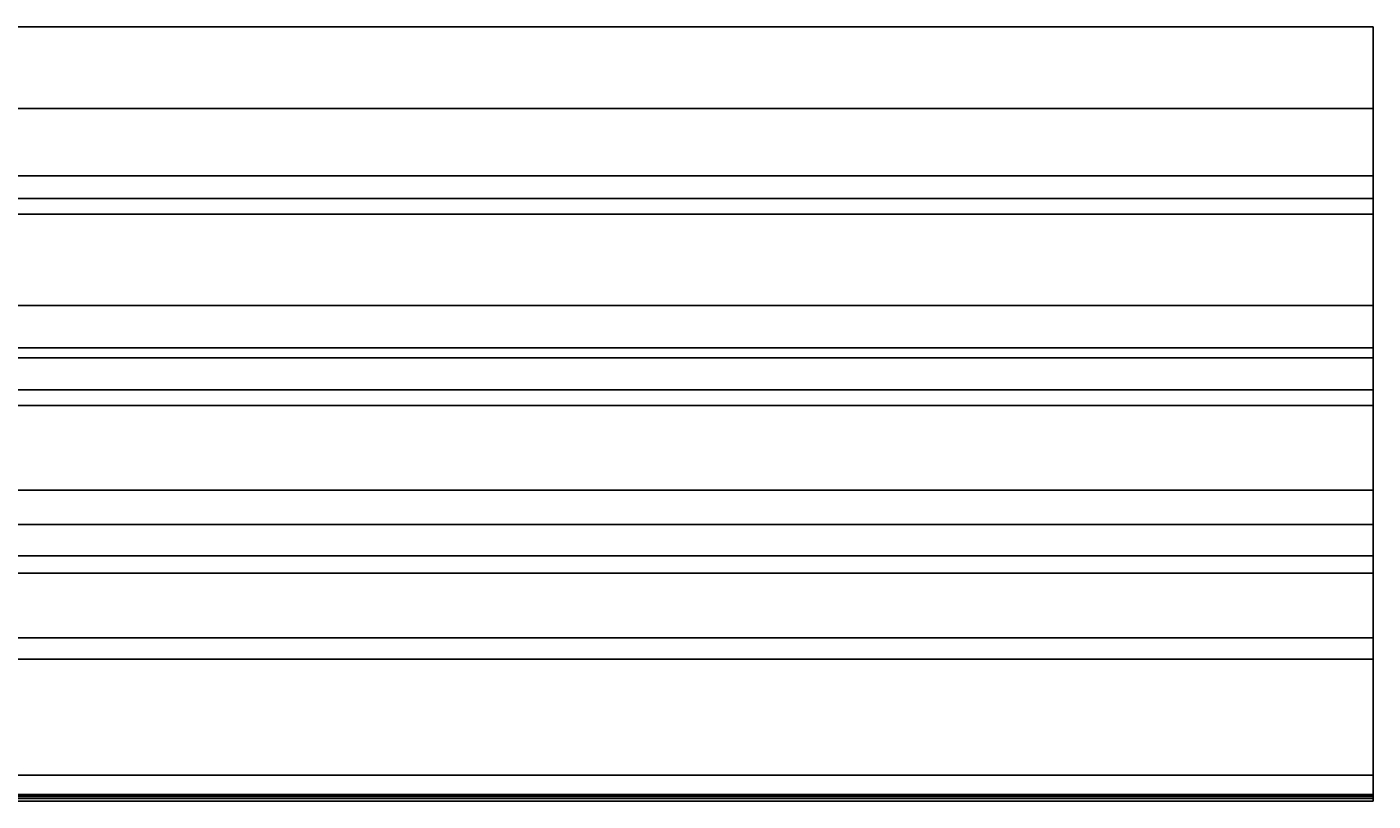
# Model space of a CAD drawing. Units: inches. Extents: x -32109 to 33221, y -19197 to 7608.
# Tile 25 of 25: x 19011 to 25711, y -2148 to 1705. Entities that reach past the tile are written whole.
import ezdxf

# ---------------------------------------------------------------- set-up
doc = ezdxf.new("R2010")
doc.units = ezdxf.units.IN
doc.header["$MEASUREMENT"] = 0
doc.layers.add('A-ANNO-DIMS', color=2, linetype='Continuous', lineweight=18)
doc.layers.add('A-ELEV', color=7, linetype='Continuous', lineweight=25)
doc.styles.get("Standard").update_dxf_attribs({"font": 'arial.ttf'})
doc.dimstyles.get("Standard").update_dxf_attribs({"dimtxt": 0.18, "dimasz": 0.18, "dimexe": 0.18, "dimexo": 0.0625, "dimgap": 0.09, "dimtad": 0, "dimtih": 1, "dimtoh": 1, "dimdec": 4, "dimzin": 0, "dimdsep": 46, "dimtxsty": 'Standard', "dimcen": 0.09, "dimadec": 0, "dimazin": 0, "dimtfac": 1, "dimtdec": 4, "dimtofl": 0, "dimtmove": 0, "dimatfit": 3, "dimfxl": 1, "dimtolj": 1, "dimtzin": 0, "dimarcsym": 0})

# ---------------------------------------------------------------- blocks, each defined once
blk = doc.blocks.new('*D11')
at = {"layer": 'A-ANNO-DIMS', "color": 0, "lineweight": -2, "transparency": 16777216}
for p, q in [((14509.6, 1705.2), (25710.6, 1705.2)), ((25710.5, 1705), (25710.5, -209.6)), ((25710.5, -2124.6), (25710.5, -210)), ((-18512.6, -2124.8), (25710.6, -2124.8))]:
    blk.add_line(p, q, dxfattribs=at)
at = {"layer": 'A-ANNO-DIMS', "color": 0, "transparency": 16777216}
for points in [[(25710.4, 1705), (25710.5, 1705), (25710.5, 1705.2)], [(25710.4, -2124.6), (25710.5, -2124.6), (25710.5, -2124.8)]]:
    blk.add_solid(points, dxfattribs=at)
at = {"layer": 'Defpoints', "color": 0, "transparency": 16777216}
for p in [(14509.6, 1705.2), (-18512.6, -2124.8), (25710.5, -2124.8)]:
    blk.add_point(p, dxfattribs=at)
at = {"layer": 'A-ANNO-DIMS', "color": 0, "transparency": 16777216, "insert": (25710.5, -209.8), "char_height": 0.18, "attachment_point": 5}
blk.add_mtext('\\A1;3830', dxfattribs=at)
blk = doc.blocks.new('*D53')
at = {"layer": 'A-ANNO-DIMS', "color": 0, "lineweight": -2, "transparency": 16777216}
for p, q in [((-9508.3, -179.7), (25710.6, -179.7)), ((25710.5, -179.9), (25710.5, -389.7)), ((25710.5, -600), (25710.5, -390.1)), ((-9508.3, -600.2), (25710.6, -600.2))]:
    blk.add_line(p, q, dxfattribs=at)
at = {"layer": 'A-ANNO-DIMS', "color": 0, "transparency": 16777216}
for points in [[(25710.4, -179.9), (25710.5, -179.9), (25710.5, -179.7)], [(25710.4, -600), (25710.5, -600), (25710.5, -600.2)]]:
    blk.add_solid(points, dxfattribs=at)
at = {"layer": 'Defpoints', "color": 0, "transparency": 16777216}
for p in [(-9508.3, -179.7), (-9508.3, -600.2), (25710.5, -600.2)]:
    blk.add_point(p, dxfattribs=at)
at = {"layer": 'A-ANNO-DIMS', "color": 0, "transparency": 16777216, "insert": (25710.5, -389.9), "char_height": 0.18, "attachment_point": 5}
blk.add_mtext('\\A1;420.5', dxfattribs=at)
blk = doc.blocks.new('*D54')
at = {"layer": 'A-ANNO-DIMS', "color": 0, "lineweight": -2, "transparency": 16777216}
for p, q in [((-9508.3, -600.2), (25710.6, -600.2)), ((25710.5, -600.3), (25710.5, -806.8)), ((25710.5, -1013.7), (25710.5, -807.2)), ((-9508.3, -1013.9), (25710.6, -1013.9))]:
    blk.add_line(p, q, dxfattribs=at)
at = {"layer": 'A-ANNO-DIMS', "color": 0, "transparency": 16777216}
for points in [[(25710.4, -600.3), (25710.5, -600.3), (25710.5, -600.2)], [(25710.4, -1013.7), (25710.5, -1013.7), (25710.5, -1013.9)]]:
    blk.add_solid(points, dxfattribs=at)
at = {"layer": 'Defpoints', "color": 0, "transparency": 16777216}
for p in [(-9508.3, -600.2), (-9508.3, -1013.9), (25710.5, -1013.9)]:
    blk.add_point(p, dxfattribs=at)
at = {"layer": 'A-ANNO-DIMS', "color": 0, "transparency": 16777216, "insert": (25710.5, -807), "char_height": 0.18, "attachment_point": 5}
blk.add_mtext('\\A1;413.7', dxfattribs=at)
blk = doc.blocks.new('*D55')
at = {"layer": 'A-ANNO-DIMS', "color": 0, "lineweight": -2, "transparency": 16777216}
for p, q in [((-9508.3, -1013.9), (25710.6, -1013.9)), ((25710.5, -1014.1), (25710.5, -1227.7)), ((25710.5, -1441.6), (25710.5, -1228)), ((-9508.3, -1441.8), (25710.6, -1441.8))]:
    blk.add_line(p, q, dxfattribs=at)
at = {"layer": 'A-ANNO-DIMS', "color": 0, "transparency": 16777216}
for points in [[(25710.4, -1014.1), (25710.5, -1014.1), (25710.5, -1013.9)], [(25710.4, -1441.6), (25710.5, -1441.6), (25710.5, -1441.8)]]:
    blk.add_solid(points, dxfattribs=at)
at = {"layer": 'Defpoints', "color": 0, "transparency": 16777216}
for p in [(-9508.3, -1013.9), (-9508.3, -1441.8), (25710.5, -1441.8)]:
    blk.add_point(p, dxfattribs=at)
at = {"layer": 'A-ANNO-DIMS', "color": 0, "transparency": 16777216, "insert": (25710.5, -1227.9), "char_height": 0.18, "attachment_point": 5}
blk.add_mtext('\\A1;427.9', dxfattribs=at)
blk = doc.blocks.new('*D56')
at = {"layer": 'A-ANNO-DIMS', "color": 0, "lineweight": -2, "transparency": 16777216}
for p, q in [((-9508.3, -1441.8), (25710.6, -1441.8)), ((25710.5, -1442), (25710.5, -1730.1)), ((25710.5, -2018.6), (25710.5, -1730.5)), ((-9508.3, -2018.8), (25710.6, -2018.8))]:
    blk.add_line(p, q, dxfattribs=at)
at = {"layer": 'A-ANNO-DIMS', "color": 0, "transparency": 16777216}
for points in [[(25710.4, -1442), (25710.5, -1442), (25710.5, -1441.8)], [(25710.4, -2018.6), (25710.5, -2018.6), (25710.5, -2018.8)]]:
    blk.add_solid(points, dxfattribs=at)
at = {"layer": 'Defpoints', "color": 0, "transparency": 16777216}
for p in [(-9508.3, -1441.8), (-9508.3, -2018.8), (25710.5, -2018.8)]:
    blk.add_point(p, dxfattribs=at)
at = {"layer": 'A-ANNO-DIMS', "color": 0, "transparency": 16777216, "insert": (25710.5, -1730.3), "char_height": 0.18, "attachment_point": 5}
blk.add_mtext('\\A1;576.9', dxfattribs=at)
blk = doc.blocks.new('*D67')
at = {"layer": 'A-ANNO-DIMS', "color": 0, "lineweight": -2, "transparency": 16777216}
for p, q in [((1645.9, 851.2), (25710.6, 851.2)), ((25710.5, 851), (25710.5, -632.3)), ((25710.5, -2116), (25710.5, -632.7)), ((1588.2, -2116.1), (25710.6, -2116.1))]:
    blk.add_line(p, q, dxfattribs=at)
at = {"layer": 'A-ANNO-DIMS', "color": 0, "transparency": 16777216}
for points in [[(25710.4, 851), (25710.5, 851), (25710.5, 851.2)], [(25710.4, -2116), (25710.5, -2116), (25710.5, -2116.1)]]:
    blk.add_solid(points, dxfattribs=at)
at = {"layer": 'Defpoints', "color": 0, "transparency": 16777216}
for p in [(1645.8, 851.2), (1588.2, -2116.1), (25710.5, -2116.1)]:
    blk.add_point(p, dxfattribs=at)
at = {"layer": 'A-ANNO-DIMS', "color": 0, "transparency": 16777216, "insert": (25710.5, -632.5), "char_height": 0.18, "attachment_point": 5}
blk.add_mtext('\\A1;2967.4', dxfattribs=at)
blk = doc.blocks.new('*D68')
at = {"layer": 'A-ANNO-DIMS', "color": 0, "lineweight": -2, "transparency": 16777216}
for p, q in [((4084.1, -927.5), (25710.6, -927.5)), ((25710.5, -927.7), (25710.5, -1521.6)), ((25710.5, -2116), (25710.5, -1522)), ((4084.1, -2116.1), (25710.6, -2116.1))]:
    blk.add_line(p, q, dxfattribs=at)
at = {"layer": 'A-ANNO-DIMS', "color": 0, "transparency": 16777216}
for points in [[(25710.4, -927.7), (25710.5, -927.7), (25710.5, -927.5)], [(25710.4, -2116), (25710.5, -2116), (25710.5, -2116.1)]]:
    blk.add_solid(points, dxfattribs=at)
at = {"layer": 'Defpoints', "color": 0, "transparency": 16777216}
for p in [(4084, -927.5), (4084, -2116.1), (25710.5, -2116.1)]:
    blk.add_point(p, dxfattribs=at)
at = {"layer": 'A-ANNO-DIMS', "color": 0, "transparency": 16777216, "insert": (25710.5, -1521.8), "char_height": 0.18, "attachment_point": 5}
blk.add_mtext('\\A1;1188.7', dxfattribs=at)
blk = doc.blocks.new('*D69')
at = {"layer": 'A-ANNO-DIMS', "color": 0, "lineweight": -2, "transparency": 16777216}
for p, q in [((5273.8, 1298.7), (25710.6, 1298.7)), ((25710.5, 1298.5), (25710.5, -411.9)), ((25710.5, -2122.6), (25710.5, -412.2)), ((5279.3, -2122.7), (25710.6, -2122.7))]:
    blk.add_line(p, q, dxfattribs=at)
at = {"layer": 'A-ANNO-DIMS', "color": 0, "transparency": 16777216}
for points in [[(25710.4, 1298.5), (25710.5, 1298.5), (25710.5, 1298.7)], [(25710.4, -2122.6), (25710.5, -2122.6), (25710.5, -2122.7)]]:
    blk.add_solid(points, dxfattribs=at)
at = {"layer": 'Defpoints', "color": 0, "transparency": 16777216}
for p in [(5273.7, 1298.7), (5279.3, -2122.7), (25710.5, -2122.7)]:
    blk.add_point(p, dxfattribs=at)
at = {"layer": 'A-ANNO-DIMS', "color": 0, "transparency": 16777216, "insert": (25710.5, -412), "char_height": 0.18, "attachment_point": 5}
blk.add_mtext('\\A1;3421.4', dxfattribs=at)
blk = doc.blocks.new('*D70')
at = {"layer": 'A-ANNO-DIMS', "color": 0, "lineweight": -2, "transparency": 16777216}
for p, q in [((8883.3, 57.8), (25710.6, 57.8)), ((25710.5, 57.6), (25710.5, -1045.1)), ((25710.5, -2148.2), (25710.5, -1045.5)), ((8832.4, -2148.4), (25710.6, -2148.4))]:
    blk.add_line(p, q, dxfattribs=at)
at = {"layer": 'A-ANNO-DIMS', "color": 0, "transparency": 16777216}
for points in [[(25710.4, 57.6), (25710.5, 57.6), (25710.5, 57.8)], [(25710.4, -2148.2), (25710.5, -2148.2), (25710.5, -2148.4)]]:
    blk.add_solid(points, dxfattribs=at)
at = {"layer": 'Defpoints', "color": 0, "transparency": 16777216}
for p in [(8883.2, 57.8), (8832.3, -2148.4), (25710.5, -2148.4)]:
    blk.add_point(p, dxfattribs=at)
at = {"layer": 'A-ANNO-DIMS', "color": 0, "transparency": 16777216, "insert": (25710.5, -1045.3), "char_height": 0.18, "attachment_point": 5}
blk.add_mtext('\\A1;2206', dxfattribs=at)
blk = doc.blocks.new('*D71')
at = {"layer": 'A-ANNO-DIMS', "color": 0, "lineweight": -2, "transparency": 16777216}
for p, q in [((11823.3, 772.8), (25710.6, 772.8)), ((25710.5, 772.6), (25710.5, 440.5)), ((25710.5, 107.9), (25710.5, 440.1)), ((11823.3, 107.7), (25710.6, 107.7))]:
    blk.add_line(p, q, dxfattribs=at)
at = {"layer": 'A-ANNO-DIMS', "color": 0, "transparency": 16777216}
for points in [[(25710.4, 772.6), (25710.5, 772.6), (25710.5, 772.8)], [(25710.4, 107.9), (25710.5, 107.9), (25710.5, 107.7)]]:
    blk.add_solid(points, dxfattribs=at)
at = {"layer": 'Defpoints', "color": 0, "transparency": 16777216}
for p in [(11823.2, 772.8), (11823.2, 107.7), (25710.5, 107.7)]:
    blk.add_point(p, dxfattribs=at)
at = {"layer": 'A-ANNO-DIMS', "color": 0, "transparency": 16777216, "insert": (25710.5, 440.3), "char_height": 0.18, "attachment_point": 5}
blk.add_mtext('\\A1;665.1', dxfattribs=at)
blk = doc.blocks.new('*D72')
at = {"layer": 'A-ANNO-DIMS', "color": 0, "lineweight": -2, "transparency": 16777216}
for p, q in [((11823.3, 107.7), (25710.6, 107.7)), ((25710.5, 107.6), (25710.5, -1004)), ((25710.5, -2116), (25710.5, -1004.4)), ((11383.7, -2116.1), (25710.6, -2116.1))]:
    blk.add_line(p, q, dxfattribs=at)
at = {"layer": 'A-ANNO-DIMS', "color": 0, "transparency": 16777216}
for points in [[(25710.4, 107.6), (25710.5, 107.6), (25710.5, 107.7)], [(25710.4, -2116), (25710.5, -2116), (25710.5, -2116.1)]]:
    blk.add_solid(points, dxfattribs=at)
at = {"layer": 'Defpoints', "color": 0, "transparency": 16777216}
for p in [(11823.2, 107.7), (11383.7, -2116.1), (25710.5, -2116.1)]:
    blk.add_point(p, dxfattribs=at)
at = {"layer": 'A-ANNO-DIMS', "color": 0, "transparency": 16777216, "insert": (25710.5, -1004.2), "char_height": 0.18, "attachment_point": 5}
blk.add_mtext('\\A1;2224', dxfattribs=at)
blk = doc.blocks.new('*D74')
at = {"layer": 'A-ANNO-DIMS', "color": 0, "lineweight": -2, "transparency": 16777216}
for p, q in [((15223.2, -771.9), (25710.6, -771.9)), ((25710.5, -772.1), (25710.5, -1053.6)), ((25710.5, -1335.5), (25710.5, -1054)), ((15223.2, -1335.7), (25710.6, -1335.7))]:
    blk.add_line(p, q, dxfattribs=at)
at = {"layer": 'A-ANNO-DIMS', "color": 0, "transparency": 16777216}
for points in [[(25710.4, -772.1), (25710.5, -772.1), (25710.5, -771.9)], [(25710.4, -1335.5), (25710.5, -1335.5), (25710.5, -1335.7)]]:
    blk.add_solid(points, dxfattribs=at)
at = {"layer": 'Defpoints', "color": 0, "transparency": 16777216}
for p in [(15223.2, -771.9), (15223.2, -1335.7), (25710.5, -1335.7)]:
    blk.add_point(p, dxfattribs=at)
at = {"layer": 'A-ANNO-DIMS', "color": 0, "transparency": 16777216, "insert": (25710.5, -1053.8), "char_height": 0.18, "attachment_point": 5}
blk.add_mtext('\\A1;563.8', dxfattribs=at)
blk = doc.blocks.new('*D75')
at = {"layer": 'A-ANNO-DIMS', "color": 0, "lineweight": -2, "transparency": 16777216}
for p, q in [((14509.6, 1705.2), (25710.6, 1705.2)), ((25710.5, 1705), (25710.5, 1012.4)), ((25710.5, 319.4), (25710.5, 1012)), ((14509.6, 319.2), (25710.6, 319.2))]:
    blk.add_line(p, q, dxfattribs=at)
at = {"layer": 'A-ANNO-DIMS', "color": 0, "transparency": 16777216}
for points in [[(25710.4, 1705), (25710.5, 1705), (25710.5, 1705.2)], [(25710.4, 319.4), (25710.5, 319.4), (25710.5, 319.2)]]:
    blk.add_solid(points, dxfattribs=at)
at = {"layer": 'Defpoints', "color": 0, "transparency": 16777216}
for p in [(14509.6, 1705.2), (14509.6, 319.2), (25710.5, 319.2)]:
    blk.add_point(p, dxfattribs=at)
at = {"layer": 'A-ANNO-DIMS', "color": 0, "transparency": 16777216, "insert": (25710.5, 1012.2), "char_height": 0.18, "attachment_point": 5}
blk.add_mtext('\\A1;1386', dxfattribs=at)
blk = doc.blocks.new('*D76')
at = {"layer": 'A-ANNO-DIMS', "color": 0, "lineweight": -2, "transparency": 16777216}
for p, q in [((16709.9, 963.7), (25710.6, 963.7)), ((25710.5, 963.5), (25710.5, 431.2)), ((25710.5, -101.4), (25710.5, 430.9)), ((15505.8, -101.6), (25710.6, -101.6))]:
    blk.add_line(p, q, dxfattribs=at)
at = {"layer": 'A-ANNO-DIMS', "color": 0, "transparency": 16777216}
for points in [[(25710.4, 963.5), (25710.5, 963.5), (25710.5, 963.7)], [(25710.4, -101.4), (25710.5, -101.4), (25710.5, -101.6)]]:
    blk.add_solid(points, dxfattribs=at)
at = {"layer": 'Defpoints', "color": 0, "transparency": 16777216}
for p in [(16709.8, 963.7), (15505.7, -101.6), (25710.5, -101.6)]:
    blk.add_point(p, dxfattribs=at)
at = {"layer": 'A-ANNO-DIMS', "color": 0, "transparency": 16777216, "insert": (25710.5, 431.1), "char_height": 0.18, "attachment_point": 5}
blk.add_mtext('\\A1;1065.3', dxfattribs=at)
blk = doc.blocks.new('*D77')
at = {"layer": 'A-ANNO-DIMS', "color": 0, "lineweight": -2, "transparency": 16777216}
for p, q in [((18109.4, -101.6), (25710.6, -101.6)), ((25710.5, -101.8), (25710.5, -1118.6)), ((25710.5, -2135.8), (25710.5, -1119)), ((18108.4, -2136), (25710.6, -2136))]:
    blk.add_line(p, q, dxfattribs=at)
at = {"layer": 'A-ANNO-DIMS', "color": 0, "transparency": 16777216}
for points in [[(25710.4, -101.8), (25710.5, -101.8), (25710.5, -101.6)], [(25710.4, -2135.8), (25710.5, -2135.8), (25710.5, -2136)]]:
    blk.add_solid(points, dxfattribs=at)
at = {"layer": 'Defpoints', "color": 0, "transparency": 16777216}
for p in [(18109.3, -101.6), (18108.4, -2136), (25710.5, -2136)]:
    blk.add_point(p, dxfattribs=at)
at = {"layer": 'A-ANNO-DIMS', "color": 0, "transparency": 16777216, "insert": (25710.5, -1118.8), "char_height": 0.18, "attachment_point": 5}
blk.add_mtext('\\A1;2034.4', dxfattribs=at)

msp = doc.modelspace()

# ---------------------------------------------------------------- linework, layer by layer
at = {"layer": 'A-ELEV'}
msp.add_line((9873.793, -2116.149), (23260.469, -2116.149), dxfattribs=at)

# ---------------------------------------------------------------- dimensions: what is measured, and where the dimension line sits
at = {"layer": 'A-ANNO-DIMS'}
for base, p1, p2, override, picture, middle in [((25710.469, -2124.791), (14509.55, 1705.162), (-18512.647, -2124.791), {"dimdec": 0, "dimlfac": 1, "dimrnd": 0, "dimzin": 0, "dimdsep": 46, "dimlunit": 2}, '*D11', (25710.469, -209.814)), ((25710.469, 319.218), (14509.55, 1705.162), (14509.55, 319.218), {"dimdec": 0, "dimlfac": 1, "dimrnd": 0, "dimzin": 0, "dimdsep": 46, "dimlunit": 2}, '*D75', (25710.469, 1012.19)), ((25710.469, -2122.749), (5273.749, 1298.671), (5279.264, -2122.749), {"dimdec": 1, "dimlfac": 1, "dimrnd": 0, "dimzin": 0, "dimdsep": 46, "dimlunit": 2}, '*D69', (25710.469, -412.039)), ((25710.469, -101.6), (16709.825, 963.73), (15505.744, -101.6), {"dimdec": 1, "dimlfac": 1, "dimrnd": 0, "dimzin": 0, "dimdsep": 46, "dimlunit": 2}, '*D76', (25710.469, 431.065)), ((25710.469, -2116.149), (1645.845, 851.205), (1588.181, -2116.149), {"dimdec": 1, "dimlfac": 1, "dimrnd": 0, "dimzin": 0, "dimdsep": 46, "dimlunit": 2}, '*D67', (25710.469, -632.472)), ((25710.469, 107.745), (11823.239, 772.828), (11823.239, 107.745), {"dimdec": 1, "dimlfac": 1, "dimrnd": 0, "dimzin": 0, "dimdsep": 46, "dimlunit": 2}, '*D71', (25710.469, 440.287)), ((25710.469, -2116.149), (11823.239, 107.745), (11383.682, -2116.149), {"dimdec": 0, "dimlfac": 1, "dimrnd": 0, "dimzin": 0, "dimdsep": 46, "dimlunit": 2}, '*D72', (25710.469, -1004.202)), ((25710.469, -2148.367), (8883.215, 57.799), (8832.289, -2148.367), {"dimdec": 0, "dimlfac": 1, "dimrnd": 0, "dimzin": 0, "dimdsep": 46, "dimlunit": 2}, '*D70', (25710.469, -1045.284)), ((25710.469, -2136.004), (18109.317, -101.6), (18108.369, -2136.004), {"dimdec": 1, "dimlfac": 1, "dimrnd": 0, "dimzin": 0, "dimdsep": 46, "dimlunit": 2}, '*D77', (25710.469, -1118.802)), ((25710.469, -600.154), (-9508.333, -179.679), (-9508.333, -600.154), {"dimdec": 1, "dimlfac": 1, "dimrnd": 0, "dimzin": 0, "dimdsep": 46, "dimlunit": 2}, '*D53', (25710.469, -389.916)), ((25710.469, -1013.888), (-9508.333, -600.154), (-9508.333, -1013.888), {"dimdec": 1, "dimlfac": 1, "dimrnd": 0, "dimzin": 0, "dimdsep": 46, "dimlunit": 2}, '*D54', (25710.469, -807.021)), ((25710.469, -1335.677), (15223.17, -771.886), (15223.17, -1335.677), {"dimdec": 1, "dimlfac": 1, "dimrnd": 0, "dimzin": 0, "dimdsep": 46, "dimlunit": 2}, '*D74', (25710.469, -1053.781)), ((25710.469, -2116.149), (4083.997, -927.479), (4083.997, -2116.149), {"dimdec": 1, "dimlfac": 1, "dimrnd": 0, "dimzin": 0, "dimdsep": 46, "dimlunit": 2}, '*D68', (25710.469, -1521.814)), ((25710.469, -1441.815), (-9508.333, -1013.888), (-9508.333, -1441.815), {"dimdec": 1, "dimlfac": 1, "dimrnd": 0, "dimzin": 0, "dimdsep": 46, "dimlunit": 2}, '*D55', (25710.469, -1227.851)), ((25710.469, -2018.754), (-9508.333, -1441.815), (-9508.333, -2018.754), {"dimdec": 1, "dimlfac": 1, "dimrnd": 0, "dimzin": 0, "dimdsep": 46, "dimlunit": 2}, '*D56', (25710.469, -1730.285))]:
    dim = msp.add_linear_dim(base=base, p1=p1, p2=p2, angle=90, dimstyle='Standard', override=override, dxfattribs=at)
    dim.commit()
    dim.dimension.update_dxf_attribs({"geometry": picture, "text_midpoint": middle})

doc.saveas('drawing.dxf')
